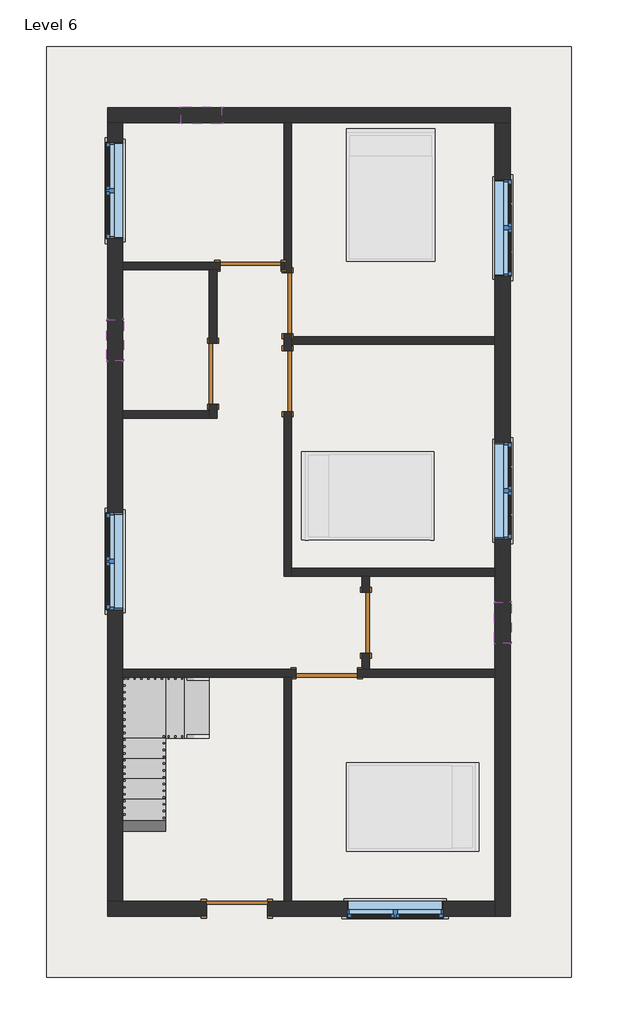
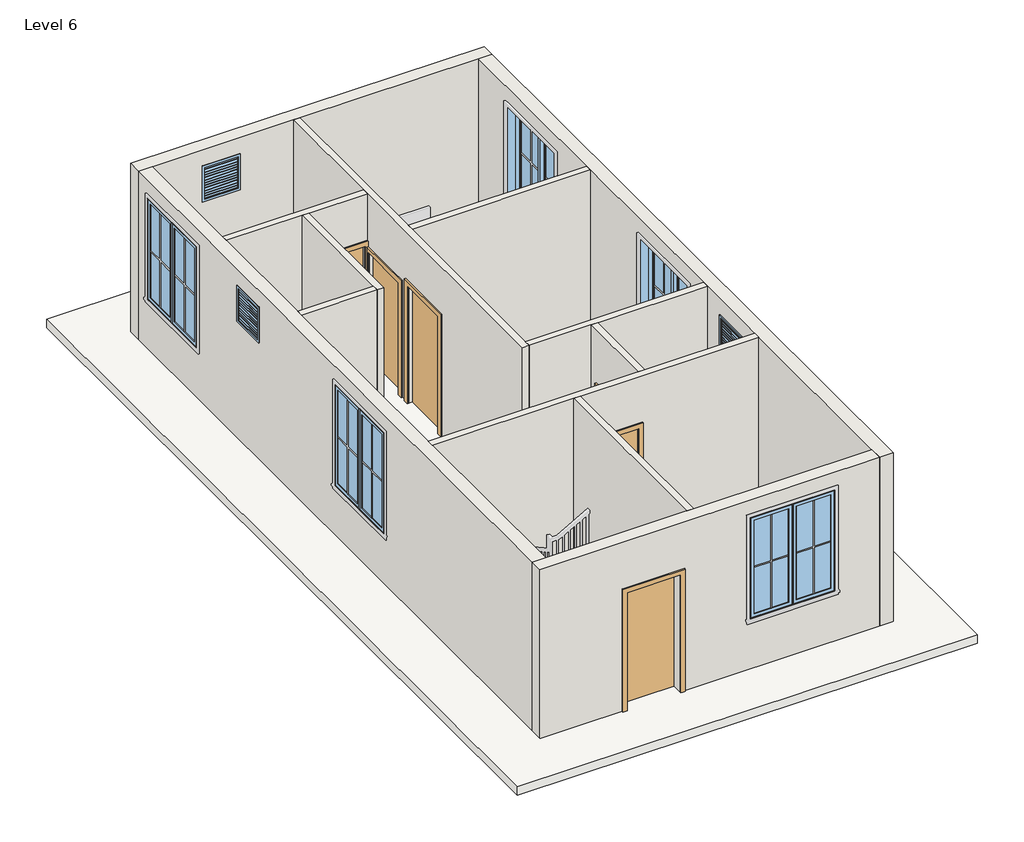
# One storey, part 1 of 2: 13 walls, 8 windows, 7 doors, 1 roof, 1 stair flight.
"""IFC4 building model written with IfcOpenShell, lengths in millimetres."""

from ifc_helpers import new_model, si_unit, frame, origin, place, context, project, spatial, polyline, outline, extrude, faceted_brep, transform, mapped, element, save
from components import door_5e62189b, door_17d80c48, door_e5f9f3c4, door_305aa2a5, door_0ca8825f, window_9ac97e1a, window_f2d8fef0

model = new_model("IFC4")

# Units and contexts
model_context = context("Model", 3, world=origin())
ifc_project = project(units=[si_unit("LENGTHUNIT", "METRE", prefix="MILLI")], contexts=[model_context])

# Site, building, storey
site = spatial("IfcSite", under=ifc_project)
building = spatial("IfcBuilding", under=site)
storey = spatial("IfcBuildingStorey", under=building, Name="Level 6", Elevation=12801.6)

# Doors
placement = place(None, origin())
door_shape = door_5e62189b(model_context)
element("IfcDoor", 1, ObjectType="Single-Flush : 36\" x 80\"", at=placement, inside=storey, context=model_context, shape_type="MappedRepresentation", body=[
    mapped(door_shape, transform((-2690.3389285, 2204.6069249, 12801.6), x_axis=(0.0, -1.0, 0.0), y_axis=(1.0, 0.0, 0.0), z_axis=(0.0, 0.0, 1.0))),
])
element("IfcDoor", 2, ObjectType="Single-Flush : 36\" x 80\"", at=placement, inside=storey, context=model_context, shape_type="MappedRepresentation", body=[
    mapped(door_shape, transform((-404.3389285, -1522.8430751, 12801.6), x_axis=(0.0, 1.0, 0.0), y_axis=(-1.0, 0.0, 0.0), z_axis=(0.0, 0.0, 1.0))),
])
door_2_shape = door_17d80c48(model_context)
element("IfcDoor", 3, ObjectType="Single-Flush : 36\" x 80\"", at=placement, inside=storey, context=model_context, shape_type="MappedRepresentation", body=[
    mapped(door_2_shape, transform((-1572.7389285, 3258.7069249, 12801.6), x_axis=(0.0, -1.0, 0.0), y_axis=(1.0, 0.0, 0.0), z_axis=(0.0, 0.0, 1.0))),
])
door_3_shape = door_e5f9f3c4(model_context)
element("IfcDoor", 4, ObjectType="Single-Flush : 36\" x 84\"", at=placement, inside=storey, context=model_context, shape_type="MappedRepresentation", body=[
    mapped(door_3_shape, transform((-2131.5389285, 3817.5069249, 12801.6), x_axis=(1.0, 0.0, 0.0), y_axis=(0.0, 1.0, 0.0), z_axis=(0.0, 0.0, 1.0))),
])
element("IfcDoor", 5, ObjectType="Single-Flush : 36\" x 84\"", at=placement, inside=storey, context=model_context, shape_type="MappedRepresentation", body=[
    mapped(door_3_shape, transform((-988.5389285, -2278.4930751, 12801.6), x_axis=(-1.0, 0.0, 0.0), y_axis=(0.0, -1.0, 0.0), z_axis=(0.0, 0.0, 1.0))),
])
door_4_shape = door_305aa2a5(model_context)
element("IfcDoor", 6, ObjectType="Single-Flush : 36\" x 84\"", at=placement, inside=storey, context=model_context, shape_type="MappedRepresentation", body=[
    mapped(door_4_shape, transform((-1572.7389285, 2090.3069249, 12801.6), x_axis=(0.0, 1.0, 0.0), y_axis=(-1.0, 0.0, 0.0), z_axis=(0.0, 0.0, 1.0))),
])
door_5_shape = door_0ca8825f(model_context)
element("IfcDoor", 7, ObjectType="Single-Flush : 36\" x 84\"", at=placement, inside=storey, context=model_context, shape_type="MappedRepresentation", body=[
    mapped(door_5_shape, transform((-2334.7389285, -5802.7430751, 12801.6), x_axis=(1.0, 0.0, 0.0), y_axis=(0.0, 1.0, 0.0), z_axis=(0.0, 0.0, 1.0))),
])

# Roof
element("IfcRoof", 8, ObjectType="ROOF 6\"", at=placement, inside=storey, context=model_context, shape_type="SweptSolid", body=[
    extrude(outline(polyline([(-5185.8889285, 7100.4569249), (2675.4110715, 7100.4569249), (2675.4110715, -6831.4430751), (-5185.8889285, -6831.4430751), (-5185.8889285, 7100.4569249)])), frame((0.0, 0.0, 12649.2), z_axis=(0.0, 0.0, 1.0), x_axis=(1.0, 0.0, 0.0)), (0.0, 0.0, 1.0), 152.4),
])

# Stair flight
element("IfcStairFlight", 9, ObjectType="3/4\" Nosing", at=placement, inside=storey, context=model_context, shape_type="Brep", body=[
    faceted_brep([(-2747.4889285, -3250.0430751, 12970.9333333), (-2747.4889285, -2335.6430751, 12970.9333333), (-3128.4889285, -2335.6430751, 12970.9333333), (-3128.4889285, -3250.0430751, 12970.9333333), (-3128.4889285, -3250.0430751, 12907.4333333), (-2754.6326785, -3250.0430751, 12907.4333333), (-2754.6326785, -2335.6430751, 12907.4333333), (-3128.4889285, -2335.6430751, 12907.4333333)], [[[0, 1, 2, 3]], [[0, 3, 4, 5]], [[2, 1, 6, 7]], [[1, 0, 5, 6]], [[4, 7, 6, 5]], [[7, 4, 3, 2]]]),
    faceted_brep([(-3128.4889285, -3250.0430751, 13140.2666667), (-3128.4889285, -2335.6430751, 13140.2666667), (-3401.5389285, -2335.6430751, 13140.2666667), (-3401.5389285, -3250.0430751, 13140.2666667), (-3401.5389285, -3250.0430751, 13076.7666667), (-3135.6326785, -3250.0430751, 13076.7666667), (-3135.6326785, -2335.6430751, 13076.7666667), (-3401.5389285, -2335.6430751, 13076.7666667)], [[[0, 1, 2, 3]], [[0, 3, 4, 5]], [[2, 1, 6, 7]], [[1, 0, 5, 6]], [[4, 7, 6, 5]], [[7, 4, 3, 2]]]),
    faceted_brep([(-3401.5389285, -3269.0930751, 13309.6), (-3401.5389285, -3250.0430751, 13309.6), (-3401.5389285, -2335.6430751, 13309.6), (-4042.8889285, -2335.6430751, 13309.6), (-4042.8889285, -3269.0930751, 13309.6), (-3401.5389285, -3269.0930751, 13246.1), (-3401.5389285, -3250.0430751, 13246.1), (-3408.6826785, -3250.0430751, 13246.1), (-3408.6826785, -2335.6430751, 13246.1), (-4042.8889285, -2335.6430751, 13246.1), (-4042.8889285, -3269.0930751, 13246.1), (-3401.5389285, -3250.0430751, 13478.9333333), (-4042.8889285, -3250.0430751, 13478.9333333), (-4042.8889285, -3285.5502386, 13478.9333333), (-4042.8889285, -3573.8930751, 13478.9333333), (-3401.5389285, -3573.8930751, 13478.9333333), (-3401.5389285, -3285.5502386, 13478.9333333), (-3401.5389285, -3573.8930751, 13406.3200976), (-3401.5389285, -3285.5502386, 13246.1), (-4042.8889285, -3285.5502386, 13246.1), (-4042.8889285, -3573.8930751, 13406.3200976), (-3401.5389285, -3554.8430751, 13648.2666667), (-4042.8889285, -3554.8430751, 13648.2666667), (-4042.8889285, -3878.6930751, 13648.2666667), (-3401.5389285, -3878.6930751, 13648.2666667), (-3401.5389285, -3878.6930751, 13575.6847552), (-4042.8889285, -3878.6930751, 13575.6847552), (-3401.5389285, -3859.6430751, 13817.6), (-4042.8889285, -3859.6430751, 13817.6), (-4042.8889285, -4183.4930751, 13817.6), (-3401.5389285, -4183.4930751, 13817.6), (-3401.5389285, -4183.4930751, 13745.0494128), (-4042.8889285, -4183.4930751, 13745.0494128), (-3401.5389285, -4164.4430751, 13986.9333333), (-4042.8889285, -4164.4430751, 13986.9333333), (-4042.8889285, -4488.2930751, 13986.9333333), (-3401.5389285, -4488.2930751, 13986.9333333), (-3401.5389285, -4488.2930751, 13914.4140703), (-4042.8889285, -4488.2930751, 13914.4140703), (-3401.5389285, -4792.8112092, 14156.2666667), (-3401.5389285, -4469.2430751, 14156.2666667), (-4042.8889285, -4469.2430751, 14156.2666667), (-4042.8889285, -4792.8112092, 14156.2666667), (-3401.5389285, -4773.7612092, 14325.6), (-3401.5389285, -5114.0119996, 14325.6), (-3401.5389285, -5114.0119996, 14262.1), (-4042.8889285, -4792.8112092, 14083.6221068), (-4042.8889285, -4773.7612092, 14325.6), (-4042.8889285, -5114.0119996, 14325.6), (-4042.8889285, -5688.4430751, 14325.6), (-3401.5389285, -5688.4430751, 14325.6), (-4042.8889285, -5114.0119996, 14262.1), (-4042.8889285, -5688.4430751, 14262.1), (-3401.5389285, -5688.4430751, 14262.1)], [[[0, 1, 2, 3, 4]], [[1, 0, 5, 6]], [[7, 1, 6]], [[3, 2, 8, 9]], [[4, 3, 9, 10]], [[11, 12, 13, 14, 15, 16]], [[0, 11, 16, 15, 17, 18, 5]], [[12, 4, 10, 19, 20, 14, 13]], [[21, 22, 23, 24]], [[21, 24, 25, 17, 15]], [[23, 22, 14, 20, 26]], [[27, 28, 29, 30]], [[27, 30, 31, 25, 24]], [[29, 28, 23, 26, 32]], [[33, 34, 35, 36]], [[33, 36, 37, 31, 30]], [[35, 34, 29, 32, 38]], [[39, 40, 41, 42]], [[39, 43, 44, 45, 37, 36, 40]], [[42, 41, 35, 38, 46]], [[43, 47, 48, 49, 50, 44]], [[47, 42, 46, 51, 52, 49, 48]], [[50, 49, 52, 53]], [[2, 1, 7, 8]], [[0, 4, 12, 11]], [[15, 14, 22, 21]], [[24, 23, 28, 27]], [[30, 29, 34, 33]], [[36, 35, 41, 40]], [[39, 42, 47, 43]], [[18, 19, 10, 9, 8, 7, 6, 5]], [[19, 18, 17, 25, 31, 37, 45, 51, 46, 38, 32, 26, 20]], [[45, 53, 52, 51]], [[53, 45, 44, 50]]]),
    faceted_brep([(-3401.5389285, -4773.7612092, 14494.9333333), (-3401.5389285, -5688.4430751, 14494.9333333), (-3128.4889285, -5688.4430751, 14494.9333333), (-3128.4889285, -4773.7612092, 14494.9333333), (-3394.3951785, -4773.7612092, 14431.4333333), (-3128.4889285, -4773.7612092, 14431.4333333), (-3394.3951785, -5688.4430751, 14431.4333333), (-3128.4889285, -5688.4430751, 14431.4333333)], [[[0, 1, 2, 3]], [[4, 0, 3, 5]], [[2, 1, 6, 7]], [[1, 0, 4, 6]], [[5, 7, 6, 4]], [[7, 5, 3, 2]]]),
    faceted_brep([(-3128.4889285, -4773.7612092, 14664.2666667), (-3128.4889285, -5688.4430751, 14664.2666667), (-2793.6303845, -5688.4430751, 14664.2666667), (-2793.6303845, -4773.7612092, 14664.2666667), (-2793.6303845, -4773.7612092, 14600.7666667), (-3121.3451785, -4773.7612092, 14600.7666667), (-3121.3451785, -5688.4430751, 14600.7666667), (-2793.6303845, -5688.4430751, 14600.7666667)], [[[0, 1, 2, 3]], [[0, 3, 4, 5]], [[2, 1, 6, 7]], [[3, 2, 7, 4]], [[1, 0, 5, 6]], [[6, 5, 4, 7]]]),
])

# Walls
element("IfcWall", 10, ObjectType="WALL 4.5\"", at=placement, inside=storey, context=model_context, shape_type="Brep", body=[
    faceted_brep([(-1629.8889285, 2801.5069249, 14833.6), (-1629.8889285, 2801.5069249, 12801.6), (-1629.8889285, 2547.5069249, 12801.6), (-1629.8889285, 2547.5069249, 14935.2), (-1629.8889285, 1633.1069249, 14935.2), (-1629.8889285, 1633.1069249, 12801.6), (-1629.8889285, -824.3430751, 12801.6), (-1629.8889285, -824.3430751, 15849.6), (-1629.8889285, 3760.3569249, 15849.6), (-1629.8889285, 3874.6569249, 15849.6), (-1629.8889285, 5957.4569249, 15849.6), (-1629.8889285, 5957.4569249, 12801.6), (-1629.8889285, 3874.6569249, 12801.6), (-1629.8889285, 3760.3569249, 12801.6), (-1629.8889285, 3715.9069249, 12801.6), (-1629.8889285, 3715.9069249, 14833.6), (-1515.5889285, 2547.5069249, 12801.6), (-1515.5889285, 2642.7569249, 12801.6), (-1515.5889285, 2757.0569249, 12801.6), (-1515.5889285, 2801.5069249, 12801.6), (-1515.5889285, 2801.5069249, 14833.6), (-1515.5889285, 3715.9069249, 14833.6), (-1515.5889285, 3715.9069249, 12801.6), (-1515.5889285, 5957.4569249, 12801.6), (-1515.5889285, 5957.4569249, 15849.6), (-1515.5889285, 2757.0569249, 15849.6), (-1515.5889285, 2642.7569249, 15849.6), (-1515.5889285, -710.0430751, 15849.6), (-1515.5889285, -824.3430751, 15849.6), (-1515.5889285, -824.3430751, 12801.6), (-1515.5889285, -710.0430751, 12801.6), (-1515.5889285, 1633.1069249, 12801.6), (-1515.5889285, 1633.1069249, 14935.2), (-1515.5889285, 2547.5069249, 14935.2)], [[[0, 1, 2, 3, 4, 5, 6, 7, 8, 9, 10, 11, 12, 13, 14, 15]], [[16, 17, 18, 19, 20, 21, 22, 23, 24, 25, 26, 27, 28, 29, 30, 31, 32, 33]], [[31, 30, 29, 6, 5]], [[2, 1, 19, 18, 17, 16]], [[14, 13, 12, 11, 23, 22]], [[11, 10, 24, 23]], [[3, 2, 16, 33]], [[4, 3, 33, 32]], [[5, 4, 32, 31]], [[20, 19, 1, 0]], [[21, 20, 0, 15]], [[22, 21, 15, 14]], [[10, 9, 8, 7, 28, 27, 26, 25, 24]], [[7, 6, 29, 28]]]),
])
element("IfcWall", 11, ObjectType="WALL 4.5\"", at=placement, inside=storey, context=model_context, shape_type="Brep", body=[
    faceted_brep([(1532.4110715, -710.0430751, 12801.6), (-1515.5889285, -710.0430751, 12801.6), (-1515.5889285, -710.0430751, 15849.6), (1532.4110715, -710.0430751, 15849.6), (1532.4110715, -824.3430751, 12801.6), (1532.4110715, -824.3430751, 15849.6), (-347.1889285, -824.3430751, 15849.6), (-461.4889285, -824.3430751, 15849.6), (-1515.5889285, -824.3430751, 15849.6), (-1515.5889285, -824.3430751, 12801.6), (-461.4889285, -824.3430751, 12801.6), (-347.1889285, -824.3430751, 12801.6)], [[[0, 1, 2, 3]], [[4, 5, 6, 7, 8, 9, 10, 11]], [[1, 0, 4, 11, 10, 9]], [[0, 3, 5, 4]], [[3, 2, 8, 7, 6, 5]], [[2, 1, 9, 8]]]),
])
element("IfcWall", 12, ObjectType="WALL 4.5\"", at=placement, inside=storey, context=model_context, shape_type="SweptSolid", body=[
    extrude(outline(polyline([(-1515.5889285, 2757.0569249), (1532.4110715, 2757.0569249), (1532.4110715, 2642.7569249), (-1515.5889285, 2642.7569249), (-1515.5889285, 2757.0569249)])), frame((0.0, 0.0, 12801.6), z_axis=(0.0, 0.0, 1.0), x_axis=(1.0, 0.0, 0.0)), (0.0, 0.0, 1.0), 3048.0),
])
element("IfcWall", 13, ObjectType="WALL 4.5\"", at=placement, inside=storey, context=model_context, shape_type="Brep", body=[
    faceted_brep([(-1674.3389285, 3760.3569249, 14935.2), (-1674.3389285, 3760.3569249, 12801.6), (-1629.8889285, 3760.3569249, 12801.6), (-1629.8889285, 3760.3569249, 15849.6), (-2633.1889285, 3760.3569249, 15849.6), (-2747.4889285, 3760.3569249, 15849.6), (-4042.8889285, 3760.3569249, 15849.6), (-4042.8889285, 3760.3569249, 12801.6), (-2747.4889285, 3760.3569249, 12801.6), (-2633.1889285, 3760.3569249, 12801.6), (-2588.7389285, 3760.3569249, 12801.6), (-2588.7389285, 3760.3569249, 14935.2), (-1629.8889285, 3874.6569249, 12801.6), (-1674.3389285, 3874.6569249, 12801.6), (-1674.3389285, 3874.6569249, 14935.2), (-2588.7389285, 3874.6569249, 14935.2), (-2588.7389285, 3874.6569249, 12801.6), (-4042.8889285, 3874.6569249, 12801.6), (-4042.8889285, 3874.6569249, 15849.6), (-1629.8889285, 3874.6569249, 15849.6)], [[[0, 1, 2, 3, 4, 5, 6, 7, 8, 9, 10, 11]], [[12, 13, 14, 15, 16, 17, 18, 19]], [[2, 1, 13, 12]], [[10, 9, 8, 7, 17, 16]], [[7, 6, 18, 17]], [[3, 2, 12, 19]], [[14, 13, 1, 0]], [[15, 14, 0, 11]], [[16, 15, 11, 10]], [[6, 5, 4, 3, 19, 18]]]),
])
element("IfcWall", 14, ObjectType="WALL 4.5\"", at=placement, inside=storey, context=model_context, shape_type="Brep", body=[
    faceted_brep([(-2747.4889285, 1747.4069249, 14833.6), (-2747.4889285, 1747.4069249, 12801.6), (-2747.4889285, 1652.1569249, 12801.6), (-2747.4889285, 1537.8569249, 12801.6), (-2747.4889285, 1537.8569249, 15849.6), (-2747.4889285, 1652.1569249, 15849.6), (-2747.4889285, 3760.3569249, 15849.6), (-2747.4889285, 3760.3569249, 12801.6), (-2747.4889285, 2661.8069249, 12801.6), (-2747.4889285, 2661.8069249, 14833.6), (-2633.1889285, 1537.8569249, 12801.6), (-2633.1889285, 1747.4069249, 12801.6), (-2633.1889285, 1747.4069249, 14833.6), (-2633.1889285, 2661.8069249, 14833.6), (-2633.1889285, 2661.8069249, 12801.6), (-2633.1889285, 3760.3569249, 12801.6), (-2633.1889285, 3760.3569249, 15849.6), (-2633.1889285, 1537.8569249, 15849.6)], [[[0, 1, 2, 3, 4, 5, 6, 7, 8, 9]], [[10, 11, 12, 13, 14, 15, 16, 17]], [[8, 7, 15, 14]], [[3, 2, 1, 11, 10]], [[7, 6, 16, 15]], [[4, 3, 10, 17]], [[12, 11, 1, 0]], [[13, 12, 0, 9]], [[14, 13, 9, 8]], [[6, 5, 4, 17, 16]]]),
])
element("IfcWall", 15, ObjectType="WALL 4.5\"", at=placement, inside=storey, context=model_context, shape_type="SweptSolid", body=[
    extrude(outline(polyline([(-4042.8889285, 1652.1569249), (-2747.4889285, 1652.1569249), (-2747.4889285, 1537.8569249), (-4042.8889285, 1537.8569249), (-4042.8889285, 1652.1569249)])), frame((0.0, 0.0, 12801.6), z_axis=(0.0, 0.0, 1.0), x_axis=(1.0, 0.0, 0.0)), (0.0, 0.0, 1.0), 3048.0),
])
element("IfcWall", 16, ObjectType="WALL 4.5\"", at=placement, inside=storey, context=model_context, shape_type="Brep", body=[
    faceted_brep([(-4042.8889285, -2335.6430751, 12801.6), (-1629.8889285, -2335.6430751, 12801.6), (-1515.5889285, -2335.6430751, 12801.6), (-1445.7389285, -2335.6430751, 12801.6), (-1445.7389285, -2335.6430751, 14935.2), (-531.3389285, -2335.6430751, 14935.2), (-531.3389285, -2335.6430751, 12801.6), (1532.4110715, -2335.6430751, 12801.6), (1532.4110715, -2335.6430751, 15849.6), (-1515.5889285, -2335.6430751, 15849.6), (-1629.8889285, -2335.6430751, 15849.6), (-4042.8889285, -2335.6430751, 15849.6), (-1445.7389285, -2221.3430751, 14935.2), (-1445.7389285, -2221.3430751, 12801.6), (-4042.8889285, -2221.3430751, 12801.6), (-4042.8889285, -2221.3430751, 15849.6), (-461.4889285, -2221.3430751, 15849.6), (-347.1889285, -2221.3430751, 15849.6), (1532.4110715, -2221.3430751, 15849.6), (1532.4110715, -2221.3430751, 12801.6), (-347.1889285, -2221.3430751, 12801.6), (-461.4889285, -2221.3430751, 12801.6), (-531.3389285, -2221.3430751, 12801.6), (-531.3389285, -2221.3430751, 14935.2)], [[[0, 1, 2, 3, 4, 5, 6, 7, 8, 9, 10, 11]], [[12, 13, 14, 15, 16, 17, 18, 19, 20, 21, 22, 23]], [[14, 13, 3, 2, 1, 0]], [[22, 21, 20, 19, 7, 6]], [[8, 7, 19, 18]], [[0, 11, 15, 14]], [[4, 3, 13, 12]], [[5, 4, 12, 23]], [[6, 5, 23, 22]], [[11, 10, 9, 8, 18, 17, 16, 15]]]),
])
element("IfcWall", 17, ObjectType="WALL 4.5\"", at=placement, inside=storey, context=model_context, shape_type="SweptSolid", body=[
    extrude(outline(polyline([(-824.3430751, 12801.6), (-1065.6430751, 12801.6), (-1065.6430751, 14833.6), (-1980.0430751, 14833.6), (-1980.0430751, 12801.6), (-2221.3430751, 12801.6), (-2221.3430751, 15849.6), (-824.3430751, 15849.6), (-824.3430751, 12801.6)])), frame((-461.4889285, 0.0, 0.0), z_axis=(1.0, 0.0, 0.0), x_axis=(0.0, 1.0, 0.0)), (0.0, 0.0, 1.0), 114.3),
])
element("IfcWall", 18, ObjectType="WALL 4.5\"", at=placement, inside=storey, context=model_context, shape_type="SweptSolid", body=[
    extrude(outline(polyline([(-1629.8889285, -5688.4430751), (-1629.8889285, -2335.6430751), (-1515.5889285, -2335.6430751), (-1515.5889285, -5688.4430751), (-1629.8889285, -5688.4430751)])), frame((0.0, 0.0, 12801.6), z_axis=(0.0, 0.0, 1.0), x_axis=(1.0, 0.0, 0.0)), (0.0, 0.0, 1.0), 3048.0),
])
element("IfcWall", 19, ObjectType="WALL 9\"", at=placement, inside=storey, context=model_context, shape_type="Brep", body=[
    faceted_brep([(-4271.4889285, 5957.4569249, 12801.6), (-4042.8889285, 5957.4569249, 12801.6), (-1629.8889285, 5957.4569249, 12801.6), (-1515.5889285, 5957.4569249, 12801.6), (1532.4110715, 5957.4569249, 12801.6), (1761.0110715, 5957.4569249, 12801.6), (1761.0110715, 5957.4569249, 15849.6), (1532.4110715, 5957.4569249, 15849.6), (-1515.5889285, 5957.4569249, 15849.6), (-1629.8889285, 5957.4569249, 15849.6), (-4042.8889285, 5957.4569249, 15849.6), (-4271.4889285, 5957.4569249, 15849.6), (-2560.1639285, 5957.4569249, 15544.8), (-2560.1639285, 5957.4569249, 14935.2), (-3169.7639285, 5957.4569249, 14935.2), (-3169.7639285, 5957.4569249, 15544.8), (-4271.4889285, 6186.0569249, 12801.6), (-4271.4889285, 6186.0569249, 15849.6), (1761.0110715, 6186.0569249, 15849.6), (1761.0110715, 6186.0569249, 12801.6), (-2560.1639285, 6186.0569249, 15544.8), (-3169.7639285, 6186.0569249, 15544.8), (-3169.7639285, 6186.0569249, 14935.2), (-2560.1639285, 6186.0569249, 14935.2)], [[[0, 1, 2, 3, 4, 5, 6, 7, 8, 9, 10, 11], [12, 13, 14, 15]], [[16, 17, 18, 19], [20, 21, 22, 23]], [[5, 4, 3, 2, 1, 0, 16, 19]], [[6, 5, 19, 18]], [[0, 11, 17, 16]], [[13, 12, 20, 23]], [[14, 13, 23, 22]], [[15, 14, 22, 21]], [[12, 15, 21, 20]], [[11, 10, 9, 8, 7, 6, 18, 17]]]),
])
element("IfcWall", 20, ObjectType="WALL 9\"", at=placement, inside=storey, context=model_context, shape_type="Brep", body=[
    faceted_brep([(1532.4110715, 5957.4569249, 12801.6), (1532.4110715, 2757.0569249, 12801.6), (1532.4110715, 2642.7569249, 12801.6), (1532.4110715, -710.0430751, 12801.6), (1532.4110715, -824.3430751, 12801.6), (1532.4110715, -2221.3430751, 12801.6), (1532.4110715, -2335.6430751, 12801.6), (1532.4110715, -5688.4430751, 12801.6), (1532.4110715, -5917.0430751, 12801.6), (1532.4110715, -5917.0430751, 15849.6), (1532.4110715, -5688.4430751, 15849.6), (1532.4110715, -2335.6430751, 15849.6), (1532.4110715, -2221.3430751, 15849.6), (1532.4110715, -824.3430751, 15849.6), (1532.4110715, -710.0430751, 15849.6), (1532.4110715, 2642.7569249, 15849.6), (1532.4110715, 2757.0569249, 15849.6), (1532.4110715, 5957.4569249, 15849.6), (1532.4110715, 3661.9319249, 15544.8), (1532.4110715, 3661.9319249, 13716.0), (1532.4110715, 5109.7319249, 13716.0), (1532.4110715, 5109.7319249, 15544.8), (1532.4110715, -271.8930751, 15544.8), (1532.4110715, -271.8930751, 13716.0), (1532.4110715, 1175.9069249, 13716.0), (1532.4110715, 1175.9069249, 15544.8), (1532.4110715, -1827.6430751, 15544.8), (1532.4110715, -1827.6430751, 14935.2), (1532.4110715, -1218.0430751, 14935.2), (1532.4110715, -1218.0430751, 15544.8), (1761.0110715, 5957.4569249, 12801.6), (1761.0110715, 5957.4569249, 15849.6), (1761.0110715, -5917.0430751, 15849.6), (1761.0110715, -5917.0430751, 12801.6), (1761.0110715, 3661.9319249, 15544.8), (1761.0110715, 5109.7319249, 15544.8), (1761.0110715, 5109.7319249, 13716.0), (1761.0110715, 3661.9319249, 13716.0), (1761.0110715, -271.8930751, 15544.8), (1761.0110715, 1175.9069249, 15544.8), (1761.0110715, 1175.9069249, 13716.0), (1761.0110715, -271.8930751, 13716.0), (1761.0110715, -1827.6430751, 15544.8), (1761.0110715, -1218.0430751, 15544.8), (1761.0110715, -1218.0430751, 14935.2), (1761.0110715, -1827.6430751, 14935.2)], [[[0, 1, 2, 3, 4, 5, 6, 7, 8, 9, 10, 11, 12, 13, 14, 15, 16, 17], [18, 19, 20, 21], [22, 23, 24, 25], [26, 27, 28, 29]], [[30, 31, 32, 33], [34, 35, 36, 37], [38, 39, 40, 41], [42, 43, 44, 45]], [[8, 7, 6, 5, 4, 3, 2, 1, 0, 30, 33]], [[0, 17, 31, 30]], [[9, 8, 33, 32]], [[19, 18, 34, 37]], [[20, 19, 37, 36]], [[21, 20, 36, 35]], [[18, 21, 35, 34]], [[23, 22, 38, 41]], [[24, 23, 41, 40]], [[25, 24, 40, 39]], [[22, 25, 39, 38]], [[27, 26, 42, 45]], [[28, 27, 45, 44]], [[29, 28, 44, 43]], [[26, 29, 43, 42]], [[17, 16, 15, 14, 13, 12, 11, 10, 9, 32, 31]]]),
])
element("IfcWall", 21, ObjectType="WALL 9\"", at=placement, inside=storey, context=model_context, shape_type="Brep", body=[
    faceted_brep([(1532.4110715, -5688.4430751, 12801.6), (-1515.5889285, -5688.4430751, 12801.6), (-1629.8889285, -5688.4430751, 12801.6), (-1877.5389285, -5688.4430751, 12801.6), (-1877.5389285, -5688.4430751, 14935.2), (-2791.9389285, -5688.4430751, 14935.2), (-2791.9389285, -5688.4430751, 12801.6), (-4042.8889285, -5688.4430751, 12801.6), (-4271.4889285, -5688.4430751, 12801.6), (-4271.4889285, -5688.4430751, 15849.6), (-4042.8889285, -5688.4430751, 15849.6), (-1629.8889285, -5688.4430751, 15849.6), (-1515.5889285, -5688.4430751, 15849.6), (1532.4110715, -5688.4430751, 15849.6), (-686.9139285, -5688.4430751, 15544.8), (-686.9139285, -5688.4430751, 13716.0), (760.8860715, -5688.4430751, 13716.0), (760.8860715, -5688.4430751, 15544.8), (-1877.5389285, -5917.0430751, 14935.2), (-1877.5389285, -5917.0430751, 12801.6), (1532.4110715, -5917.0430751, 12801.6), (1532.4110715, -5917.0430751, 15849.6), (-4271.4889285, -5917.0430751, 15849.6), (-4271.4889285, -5917.0430751, 12801.6), (-2791.9389285, -5917.0430751, 12801.6), (-2791.9389285, -5917.0430751, 14935.2), (-686.9139285, -5917.0430751, 15544.8), (760.8860715, -5917.0430751, 15544.8), (760.8860715, -5917.0430751, 13716.0), (-686.9139285, -5917.0430751, 13716.0)], [[[0, 1, 2, 3, 4, 5, 6, 7, 8, 9, 10, 11, 12, 13], [14, 15, 16, 17]], [[18, 19, 20, 21, 22, 23, 24, 25], [26, 27, 28, 29]], [[24, 23, 8, 7, 6]], [[20, 19, 3, 2, 1, 0]], [[0, 13, 21, 20]], [[9, 8, 23, 22]], [[15, 14, 26, 29]], [[16, 15, 29, 28]], [[17, 16, 28, 27]], [[14, 17, 27, 26]], [[4, 3, 19, 18]], [[5, 4, 18, 25]], [[6, 5, 25, 24]], [[13, 12, 11, 10, 9, 22, 21]]]),
])
element("IfcWall", 22, ObjectType="WALL 9\"", at=placement, inside=storey, context=model_context, shape_type="Brep", body=[
    faceted_brep([(-4042.8889285, -5688.4430751, 12801.6), (-4042.8889285, -2335.6430751, 12801.6), (-4042.8889285, -2221.3430751, 12801.6), (-4042.8889285, 1537.8569249, 12801.6), (-4042.8889285, 1652.1569249, 12801.6), (-4042.8889285, 3760.3569249, 12801.6), (-4042.8889285, 3874.6569249, 12801.6), (-4042.8889285, 5957.4569249, 12801.6), (-4042.8889285, 5957.4569249, 15849.6), (-4042.8889285, 3874.6569249, 15849.6), (-4042.8889285, 3760.3569249, 15849.6), (-4042.8889285, 1652.1569249, 15849.6), (-4042.8889285, 1537.8569249, 15849.6), (-4042.8889285, -2221.3430751, 15849.6), (-4042.8889285, -2335.6430751, 15849.6), (-4042.8889285, -5688.4430751, 15849.6), (-4042.8889285, 5668.5319249, 15544.8), (-4042.8889285, 5668.5319249, 13716.0), (-4042.8889285, 4220.7319249, 13716.0), (-4042.8889285, 4220.7319249, 15544.8), (-4042.8889285, 121.8069249, 15544.8), (-4042.8889285, 121.8069249, 13716.0), (-4042.8889285, -1325.9930751, 13716.0), (-4042.8889285, -1325.9930751, 15544.8), (-4042.8889285, 2401.4569249, 15544.8), (-4042.8889285, 3011.0569249, 15544.8), (-4042.8889285, 3011.0569249, 14935.2), (-4042.8889285, 2401.4569249, 14935.2), (-4271.4889285, -5688.4430751, 12801.6), (-4271.4889285, -5688.4430751, 15849.6), (-4271.4889285, 5957.4569249, 15849.6), (-4271.4889285, 5957.4569249, 12801.6), (-4271.4889285, 5668.5319249, 15544.8), (-4271.4889285, 4220.7319249, 15544.8), (-4271.4889285, 4220.7319249, 13716.0), (-4271.4889285, 5668.5319249, 13716.0), (-4271.4889285, 121.8069249, 15544.8), (-4271.4889285, -1325.9930751, 15544.8), (-4271.4889285, -1325.9930751, 13716.0), (-4271.4889285, 121.8069249, 13716.0), (-4271.4889285, 2401.4569249, 15544.8), (-4271.4889285, 2401.4569249, 14935.2), (-4271.4889285, 3011.0569249, 14935.2), (-4271.4889285, 3011.0569249, 15544.8)], [[[0, 1, 2, 3, 4, 5, 6, 7, 8, 9, 10, 11, 12, 13, 14, 15], [16, 17, 18, 19], [20, 21, 22, 23], [24, 25, 26, 27]], [[28, 29, 30, 31], [32, 33, 34, 35], [36, 37, 38, 39], [40, 41, 42, 43]], [[7, 6, 5, 4, 3, 2, 1, 0, 28, 31]], [[0, 15, 29, 28]], [[8, 7, 31, 30]], [[17, 16, 32, 35]], [[18, 17, 35, 34]], [[19, 18, 34, 33]], [[16, 19, 33, 32]], [[21, 20, 36, 39]], [[22, 21, 39, 38]], [[23, 22, 38, 37]], [[20, 23, 37, 36]], [[41, 40, 24, 27]], [[42, 41, 27, 26]], [[43, 42, 26, 25]], [[40, 43, 25, 24]], [[15, 14, 13, 12, 11, 10, 9, 8, 30, 29]]]),
])

# Windows
window_shape = window_9ac97e1a(model_context)
element("IfcWindow", 23, ObjectType="Window-Casement-Double : 57\" x 72\"", at=placement, inside=storey, context=model_context, shape_type="MappedRepresentation", body=[
    mapped(window_shape, transform((-4157.1889285, 4944.6319249, 12801.6), x_axis=(0.0, 1.0, 0.0), y_axis=(-1.0, 0.0, 0.0), z_axis=(0.0, 0.0, 1.0))),
])
element("IfcWindow", 24, ObjectType="Window-Casement-Double : 57\" x 72\"", at=placement, inside=storey, context=model_context, shape_type="MappedRepresentation", body=[
    mapped(window_shape, transform((1646.7110715, 4385.8319249, 12801.6), x_axis=(0.0, -1.0, 0.0), y_axis=(1.0, 0.0, 0.0), z_axis=(0.0, 0.0, 1.0))),
])
element("IfcWindow", 25, ObjectType="Window-Casement-Double : 57\" x 72\"", at=placement, inside=storey, context=model_context, shape_type="MappedRepresentation", body=[
    mapped(window_shape, transform((-4157.1889285, -602.0930751, 12801.6), x_axis=(0.0, 1.0, 0.0), y_axis=(-1.0, 0.0, 0.0), z_axis=(0.0, 0.0, 1.0))),
])
element("IfcWindow", 26, ObjectType="Window-Casement-Double : 57\" x 72\"", at=placement, inside=storey, context=model_context, shape_type="MappedRepresentation", body=[
    mapped(window_shape, transform((1646.7110715, 452.0069249, 12801.6), x_axis=(0.0, -1.0, 0.0), y_axis=(1.0, 0.0, 0.0), z_axis=(0.0, 0.0, 1.0))),
])
element("IfcWindow", 27, ObjectType="Window-Casement-Double : 57\" x 72\"", at=placement, inside=storey, context=model_context, shape_type="MappedRepresentation", body=[
    mapped(window_shape, transform((36.9860715, -5802.7430751, 12801.6), x_axis=(-1.0, 0.0, 0.0), y_axis=(0.0, -1.0, 0.0), z_axis=(0.0, 0.0, 1.0))),
])
window_2_shape = window_f2d8fef0(model_context)
element("IfcWindow", 28, ObjectType="Window-Louvers : 24\" x 24\"", at=placement, inside=storey, context=model_context, shape_type="MappedRepresentation", body=[
    mapped(window_2_shape, transform((-2864.9639285, 6065.4069249, 14020.8), x_axis=(-1.0, 0.0, 0.0), y_axis=(0.0, -1.0, 0.0), z_axis=(0.0, 0.0, 1.0))),
])
element("IfcWindow", 29, ObjectType="Window-Louvers : 24\" x 24\"", at=placement, inside=storey, context=model_context, shape_type="MappedRepresentation", body=[
    mapped(window_2_shape, transform((-4163.5389285, 2706.2569249, 14020.8), x_axis=(0.0, 1.0, 0.0), y_axis=(-1.0, 0.0, 0.0), z_axis=(0.0, 0.0, 1.0))),
])
element("IfcWindow", 30, ObjectType="Window-Louvers : 24\" x 24\"", at=placement, inside=storey, context=model_context, shape_type="MappedRepresentation", body=[
    mapped(window_2_shape, transform((1640.3610715, -1522.8430751, 14020.8), x_axis=(0.0, 1.0, 0.0), y_axis=(-1.0, 0.0, 0.0), z_axis=(0.0, 0.0, 1.0))),
])

save(model, "model.ifc")

# Revit data of these elements
# Type "Single-Flush : 36\" x 80\""
#   Type Mark = "6"
#   Construction Type Id = "MDOOR"
#   Assembly Code = "C1020"
#   Analytic Construction = "Metal"
#   Thickness = 0' - 2"
#   Heat Transfer Coefficient (U) = 0.651978 BTU/(h·ft²·°F)
#   Height = 6' - 8"
#   Trim Projection Ext = 0' - 1"
#   Trim Projection Int = 0' - 1"
#   Trim Width = 0' - 3"
#   Width = 3' - 0"
#   Define Thermal Properties by = 1
#   Define Thermal Properties by = 1
#   Door Material = Door - Panel
#   Frame Material = Door - Frame
#   Visual Light Transmittance = 0
#   Solar Heat Gain Coefficient = 0
#   Function = (empty or 0)
#   Wall Closure = (empty or 0)
# Type "Single-Flush : 36\" x 84\""
#   Type Mark = "1"
#   Construction Type Id = "MDOOR"
#   Assembly Code = "C1020"
#   Analytic Construction = "Metal"
#   Thickness = 0' - 2"
#   Heat Transfer Coefficient (U) = 0.651978 BTU/(h·ft²·°F)
#   Height = 7' - 0"
#   Trim Projection Ext = 0' - 1"
#   Trim Projection Int = 0' - 1"
#   Trim Width = 0' - 3"
#   Width = 3' - 0"
#   Define Thermal Properties by = 1
#   Define Thermal Properties by = 1
#   Door Material = Door - Panel
#   Frame Material = Door - Frame
#   Visual Light Transmittance = 0
#   Solar Heat Gain Coefficient = 0
#   Function = (empty or 0)
#   Wall Closure = (empty or 0)
# Type "ROOF 6\""
#   Assembly Code = "B1020"
#   Layers, outside or top first: 0' - 6" no material (function 1)
# Type "WALL 4.5\""
#   Assembly Code = "B2010"
#   Layers, outside or top first: 0' - 4 1/2" no material (function 1)
# Type "WALL 9\""
#   Assembly Code = "B2010"
#   Layers, outside or top first: 0' - 9" no material (function 1)
# Type "Window-Casement-Double : 57\" x 72\""
#   Type Mark = "17"
#   Fire Rating = "0.5h"
#   Assembly Code = "B2020100"
#   Analytic Construction = "Double glazing - domestic"
#   Frame Extension [instance default] = 0' - 0 1/4"
#   Window Inset [instance default] = 0' - 0"
#   Wall Thickness [instance default] = 0' - 6"
#   Interior Wall Closure [instance default] = 0' - 2 1/4"
#   Half Width = 2' - 4 1/2"
#   Visual Light Transmittance = 0.81
#   Thermal Resistance (R) = 1.8146 (h·ft²·°F)/BTU
#   Solar Heat Gain Coefficient = 0.76
#   Rough Width = 4' - 9 1/2"
#   Rough Height = 6' - 0 1/2"
#   Height = 6' - 0"
#   Heat Transfer Coefficient (U) = 0.5511 BTU/(h·ft²·°F)
#   Exterior Wall Closure [instance default] = 0' - 1 1/4"
#   Extension Jamb [instance default] = 0' - 2 1/4"
#   Default Sill Height = 3' - 0"
#   Width = 4' - 9"
#   Define Thermal Properties by = 0
#   Muntin Visibility = yes
#   Interior Trim Visibility [instance default] = yes
#   Exterior Trim Visibility [instance default] = yes
#   Extension Jamb Visibility [instance default] = yes
#   Interior Trim Material = Wood - Stained
#   Muntin Pattern = Muntin Pattern_2x2 : Muntin Pattern_2x2
#   Interior Trim = Trim-Window-Interior-Flat : Picture Frame
#   Interior Frame Material = Wood - Stained
#   Glass Panel Material = Glass
#   Exterior Trim Material = Clad - White
#   Exterior Trim = Trim-Window-Exterior-Flat : with Sill
#   Exterior Frame Material = Clad - White
#   Wall Closure = (empty or 0)
# Type "Window-Louvers : 24\" x 24\""
#   Type Mark = "18"
#   Construction Type Id = "GSP4R"
#   Assembly Code = "B20"
#   Analytic Construction = "1/8 in Pilkington single glazing"
#   Visual Light Transmittance = 0.9
#   Thermal Resistance (R) = 1.53941 (h·ft²·°F)/BTU
#   Solar Heat Gain Coefficient = 0.78
#   Max Height = 1' - 11.74264"
#   Height = 2' - 0"
#   Heat Transfer Coefficient (U) = 0.6496 BTU/(h·ft²·°F)
#   Blade Width [instance default] = 1' - 10 1/2"
#   Blade Vertical Thickness = 0' - 0.35355"
#   Blade Thickness = 0' - 0 1/4"
#   Blade Spacing = 0' - 1 1/2"
#   Blade Height = 0' - 1.85355"
#   Blade Depth = 0' - 3"
#   Blade Angle = 45.00°
#   Default Sill Height = 3' - 0"
#   Trim Projection_Exterior = 0' - 0 1/2"
#   Trim Projection_Interior = 0' - 0 1/2"
#   Trim Width_Exterior = 0' - 1 1/2"
#   Trim Width_Interior = 0' - 1 1/2"
#   Width = 2' - 0"
#   Max Blade Count = 12
#   Define Thermal Properties by = 1
#   Blade Count = 12
#   Frame Material = Birch
#   Louver Material = Birch
#   Trim Exterior Material = Birch
#   Trim Interior Material = Birch
#   Wall Closure = (empty or 0)
# Elements 1, 2, 3 (IfcDoor, "Single-Flush : 36\" x 80\"")
#   Phase Created = New Construction
#   Materials on its faces: "Door - Frame", "Door - Panel"
# Elements 4, 5, 6, 7 (IfcDoor, "Single-Flush : 36\" x 84\"")
#   Phase Created = New Construction
#   Materials on its faces: "Door - Frame", "Door - Panel"
# Element 8 (IfcRoof, "ROOF 6\"")
#   built-in parameter 1001705 = 42 (stored number, unit not read)
#   built-in parameter 1001701 = -0.5 (stored number, unit not read)
#   built-in parameter 1001710 = 33615
#   Phase Created = New Construction
#   Materials on its faces: "Default Roof", "Door - Panel"
# Element 9 (IfcStairFlight, "3/4\" Nosing")
#   Phase Created = New Construction
#   Materials on its faces: "Concrete, Cast-in-Place gray"
# Elements 10, 11, 12, 13, 14, 15, 16, 17, 18 (IfcWall, "WALL 4.5\"")
#   Top Offset = 0' - 0"
#   Base Offset = 0' - 0"
#   Unconnected Height = 10' - 0"
#   wall height = 10' - 0"
#   Phase Created = New Construction
#   Base Constraint = Level 6
#   Materials on its faces: "Default Wall"
# Elements 19, 20, 21, 22 (IfcWall, "WALL 9\"")
#   Top Offset = 0' - 0"
#   Base Offset = 0' - 0"
#   Unconnected Height = 10' - 0"
#   wall height = 10' - 0"
#   Phase Created = New Construction
#   Base Constraint = Level 6
#   Materials on its faces: "Default Wall", "Copper"
# Element 23 (IfcWindow, "Window-Casement-Double : 57\" x 72\"")
#   Mark = "33"
#   Window Inset = 0' - 0"
#   Interior Wall Closure = 0' - 2 1/4"
#   Frame Extension = 0' - 0 1/4"
#   Exterior Wall Closure = 0' - 1 1/4"
#   Interior Trim Visibility = yes
#   Exterior Trim Visibility = yes
#   Phase Created = New Construction
#   Materials on its faces: "Wood - Stained", "Glass", "Clad - White"
# Element 24 (IfcWindow, "Window-Casement-Double : 57\" x 72\"")
#   Mark = "34"
#   Window Inset = 0' - 0"
#   Interior Wall Closure = 0' - 2 1/4"
#   Frame Extension = 0' - 0 1/4"
#   Exterior Wall Closure = 0' - 1 1/4"
#   Interior Trim Visibility = yes
#   Exterior Trim Visibility = yes
#   Phase Created = New Construction
#   Materials on its faces: "Wood - Stained", "Glass", "Clad - White"
# Element 25 (IfcWindow, "Window-Casement-Double : 57\" x 72\"")
#   Mark = "35"
#   Window Inset = 0' - 0"
#   Interior Wall Closure = 0' - 2 1/4"
#   Frame Extension = 0' - 0 1/4"
#   Exterior Wall Closure = 0' - 1 1/4"
#   Interior Trim Visibility = yes
#   Exterior Trim Visibility = yes
#   Phase Created = New Construction
#   Materials on its faces: "Wood - Stained", "Glass", "Clad - White"
# Element 26 (IfcWindow, "Window-Casement-Double : 57\" x 72\"")
#   Mark = "36"
#   Window Inset = 0' - 0"
#   Interior Wall Closure = 0' - 2 1/4"
#   Frame Extension = 0' - 0 1/4"
#   Exterior Wall Closure = 0' - 1 1/4"
#   Interior Trim Visibility = yes
#   Exterior Trim Visibility = yes
#   Phase Created = New Construction
#   Materials on its faces: "Wood - Stained", "Glass", "Clad - White"
# Element 27 (IfcWindow, "Window-Casement-Double : 57\" x 72\"")
#   Mark = "37"
#   Window Inset = 0' - 0"
#   Interior Wall Closure = 0' - 2 1/4"
#   Frame Extension = 0' - 0 1/4"
#   Exterior Wall Closure = 0' - 1 1/4"
#   Interior Trim Visibility = yes
#   Exterior Trim Visibility = yes
#   Phase Created = New Construction
#   Materials on its faces: "Wood - Stained", "Glass", "Clad - White"
# Element 28 (IfcWindow, "Window-Louvers : 24\" x 24\"")
#   Mark = "38"
#   Blade Width = 1' - 10 1/2"
#   Phase Created = New Construction
#   Materials on its faces: "Birch"
# Element 29 (IfcWindow, "Window-Louvers : 24\" x 24\"")
#   Mark = "39"
#   Blade Width = 1' - 10 1/2"
#   Phase Created = New Construction
#   Materials on its faces: "Birch"
# Element 30 (IfcWindow, "Window-Louvers : 24\" x 24\"")
#   Mark = "40"
#   Blade Width = 1' - 10 1/2"
#   Phase Created = New Construction
#   Materials on its faces: "Birch"
# Materials
#   "Door - Panel": class "Wood", colour RGB 210 159 95, transparency 0, Cost = 0
#   "Door - Frame": colour RGB 118 70 51, transparency 0, Cost = 0
#   "Wood - Stained": class "Wood", colour RGB 224 178 126, transparency 0, Cost = 0
#   "Glass": class "Glass", colour RGB 0 128 192, transparency 0.75, Description = "Soda Lime Glass", Cost = 0
#   "Clad - White": class "Wood", colour RGB 242 242 238, transparency 0, Cost = 0
#   "Birch": class "Wood", colour RGB 224 178 126, transparency 0, Description = "Betula Alleghaniensis", Cost = 0
#   "Default Roof": colour RGB 88 101 114, transparency 0, Cost = 0
#   "Concrete, Cast-in-Place gray": class "Concrete", colour RGB 192 192 192, transparency 0, Description = "Cast-in-place concrete", Cost = 0
#   "Default Wall": colour RGB 128 128 128, transparency 0, Cost = 0
#   "Copper": class "Metal", colour RGB 0 0 0, transparency 0, Description = "Copper, matte finish", Cost = 0
